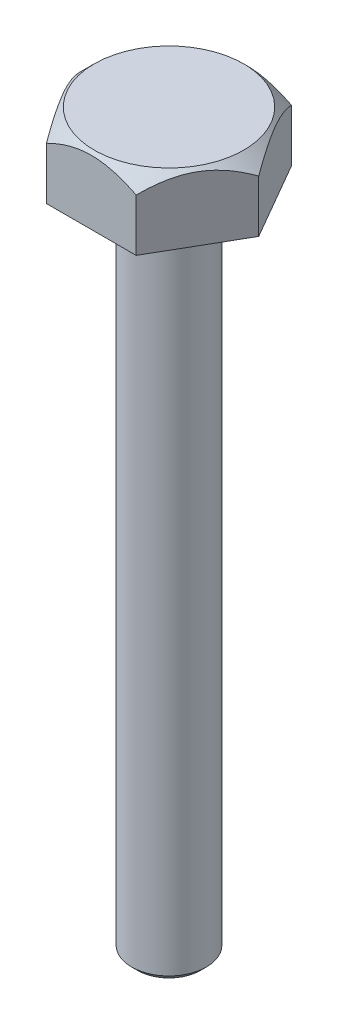
ISO-10303-21;
HEADER;
FILE_DESCRIPTION(('STEP AP214'),'2;1');
FILE_NAME('part.step','',(''),(''),'','','');
FILE_SCHEMA(('AUTOMOTIVE_DESIGN { 1 0 10303 214 1 1 1 1 }'));
ENDSEC;
DATA;
#1=APPLICATION_CONTEXT('core data for automotive mechanical design processes');
#2=APPLICATION_PROTOCOL_DEFINITION('international standard','automotive_design',2000,#1);
#3=PRODUCT_CONTEXT('',#1,'mechanical');
#4=PRODUCT('Part','Part','',(#3));
#5=PRODUCT_RELATED_PRODUCT_CATEGORY('part','',(#4));
#6=PRODUCT_DEFINITION_FORMATION('','',#4);
#7=PRODUCT_DEFINITION_CONTEXT('part definition',#1,'design');
#8=PRODUCT_DEFINITION('design','',#6,#7);
#9=PRODUCT_DEFINITION_SHAPE('','',#8);
#10=(LENGTH_UNIT() NAMED_UNIT(*) SI_UNIT(.MILLI.,.METRE.));
#11=(NAMED_UNIT(*) PLANE_ANGLE_UNIT() SI_UNIT($,.RADIAN.));
#12=(NAMED_UNIT(*) SI_UNIT($,.STERADIAN.) SOLID_ANGLE_UNIT());
#13=UNCERTAINTY_MEASURE_WITH_UNIT(LENGTH_MEASURE(1.E-05),#10,'distance_accuracy_value','');
#14=(GEOMETRIC_REPRESENTATION_CONTEXT(3) GLOBAL_UNCERTAINTY_ASSIGNED_CONTEXT((#13)) GLOBAL_UNIT_ASSIGNED_CONTEXT((#10,
#11,#12)) REPRESENTATION_CONTEXT('',''));
#15=CARTESIAN_POINT('',(0.,0.,0.));
#16=DIRECTION('',(0.,0.,1.));
#17=DIRECTION('',(1.,0.,0.));
#18=AXIS2_PLACEMENT_3D('',#15,#16,#17);
#19=CARTESIAN_POINT('',(30.0222139978612,-45.,51.9999999999998));
#20=DIRECTION('',(0.866025403784441,0.,0.499999999999995));
#21=DIRECTION('',(0.499999999999995,0.,-0.866025403784442));
#22=AXIS2_PLACEMENT_3D('',#19,#20,#21);
#23=PLANE('',#22);
#24=DIRECTION('',(0.,1.,0.));
#25=VECTOR('',#24,1.);
#26=CARTESIAN_POINT('',(60.0444279957212,-45.,0.));
#27=LINE('',#26,#25);
#28=CARTESIAN_POINT('',(60.0444279957212,-45.,0.));
#29=VERTEX_POINT('',#28);
#30=CARTESIAN_POINT('',(60.0444279957212,-10.0000000000014,0.));
#31=VERTEX_POINT('',#30);
#32=EDGE_CURVE('E126',#29,#31,#27,.T.);
#33=ORIENTED_EDGE('',*,*,#32,.T.);
#34=CARTESIAN_POINT('',(60.0445434657751,-10.0001154703869,-0.0002));
#35=CARTESIAN_POINT('',(59.7864654589408,-9.74204102394825,0.446804220153159));
#36=CARTESIAN_POINT('',(59.5273934547252,-9.4879536627119,0.895530094273221));
#37=CARTESIAN_POINT('',(59.007180391372,-8.98833098939079,1.79656555076206));
#38=CARTESIAN_POINT('',(58.7460392258412,-8.74279612061098,2.24887531740909));
#39=CARTESIAN_POINT('',(57.9591776962599,-8.01969424317608,3.61175946516538));
#40=CARTESIAN_POINT('',(57.4302681129248,-7.5558800497852,4.52785773611185));
#41=CARTESIAN_POINT('',(56.3606292168537,-6.66782291766471,6.38052664985892));
#42=CARTESIAN_POINT('',(55.8198495703374,-6.24382173529158,7.31718447332428));
#43=CARTESIAN_POINT('',(54.7294034599511,-5.44455349422062,9.20589253942921));
#44=CARTESIAN_POINT('',(54.1797383691726,-5.06927898510395,10.1579404038045));
#45=CARTESIAN_POINT('',(53.0804089118776,-4.37937556292623,12.0620348780967));
#46=CARTESIAN_POINT('',(52.5308802486714,-4.06388637101252,13.0138464429852));
#47=CARTESIAN_POINT('',(51.4240281951886,-3.49267453957314,14.9309704360794));
#48=CARTESIAN_POINT('',(50.8667044235457,-3.23695483511355,15.8962835248308));
#49=CARTESIAN_POINT('',(49.7467987752483,-2.79178958670772,17.8360170073652));
#50=CARTESIAN_POINT('',(49.1842323235144,-2.60218978873854,18.8104106844021));
#51=CARTESIAN_POINT('',(48.0543060242163,-2.2934501655637,20.7675004435948));
#52=CARTESIAN_POINT('',(47.4869469056895,-2.17429981294089,21.7501952630207));
#53=CARTESIAN_POINT('',(46.5113427741717,-2.03319122911529,23.4399911868836));
#54=CARTESIAN_POINT('',(46.1037295403586,-1.99322993327754,24.1459980176853));
#55=CARTESIAN_POINT('',(45.288020597666,-1.95167612563039,25.5588473506173));
#56=CARTESIAN_POINT('',(44.8799249140734,-1.95008168491468,26.2656898089493));
#57=CARTESIAN_POINT('',(44.0640057964976,-1.98529951069165,27.6789031754573));
#58=CARTESIAN_POINT('',(43.6561825137942,-2.02212562962843,28.3852738216091));
#59=CARTESIAN_POINT('',(42.8418298899032,-2.13363679445459,29.7957739414654));
#60=CARTESIAN_POINT('',(42.4353005710197,-2.20832248941607,30.4999033765379));
#61=CARTESIAN_POINT('',(41.623922764868,-2.39454189299686,31.9052509609266));
#62=CARTESIAN_POINT('',(41.2190765583396,-2.50611518507183,32.6064651598853));
#63=CARTESIAN_POINT('',(40.412216092256,-2.76451095087709,34.0039884817607));
#64=CARTESIAN_POINT('',(40.0102018479483,-2.9113336142421,34.7002975782681));
#65=CARTESIAN_POINT('',(39.2096518497491,-3.23827454574057,36.0868908491484));
#66=CARTESIAN_POINT('',(38.8111155333365,-3.41838732093504,36.7771759978363));
#67=CARTESIAN_POINT('',(38.017875656152,-3.80977115977922,38.1511077677096));
#68=CARTESIAN_POINT('',(37.6231724061646,-4.02104472782916,38.8347538506002));
#69=CARTESIAN_POINT('',(36.6070287630477,-4.60521339166235,40.594766268267));
#70=CARTESIAN_POINT('',(35.9887304273657,-5.00009639499698,41.6656903999035));
#71=CARTESIAN_POINT('',(34.7633032405128,-5.85344879079695,43.7881925485089));
#72=CARTESIAN_POINT('',(34.1561747269537,-6.31192010167665,44.8397699807171));
#73=CARTESIAN_POINT('',(32.9548834468553,-7.28227147123561,46.9204675125369));
#74=CARTESIAN_POINT('',(32.3606866497277,-7.79398356114847,47.9496465548567));
#75=CARTESIAN_POINT('',(31.4776043881334,-8.59647147709582,49.4791898992009));
#76=CARTESIAN_POINT('',(31.1846889985081,-8.86971037589588,49.9865342363506));
#77=CARTESIAN_POINT('',(30.6014667479989,-9.42700542859909,50.9967048063374));
#78=CARTESIAN_POINT('',(30.3111597002235,-9.71106079972311,51.4995313628796));
#79=CARTESIAN_POINT('',(30.0220985278074,-10.0001154703873,52.0001999999998));
#80=B_SPLINE_CURVE_WITH_KNOTS('',3,(#34,#35,#36,#37,#38,#39,#40,#41,#42,#43,#44,#45,#46,#47,#48,
#49,#50,#51,#52,#53,#54,#55,#56,#57,#58,#59,#60,#61,#62,#63,#64,#65,#66,#67,#68,#69,#70,#71,#72,
#73,#74,#75,#76,#77,#78,#79),.UNSPECIFIED.,.F.,.F.,(4,2,2,2,2,2,2,2,2,2,2,2,2,2,2,2,2,2,2,2,2,2,
4),(0.,1.73120255917824,3.46249471937635,6.92674897903945,10.410836798543,13.8943912642053,
17.3232079778031,20.7521930329857,24.1731240857036,27.5935438118118,30.0413233219973,
32.4889797690031,34.9375190179701,37.3861002466015,39.8373175810706,42.2885481029042,
44.7393745269946,47.1903980320212,51.0825946301753,54.974908678706,58.8552952790946,
60.7944610079078,62.7334866666266),.UNSPECIFIED.);
#81=CARTESIAN_POINT('',(30.0222139978612,-10.0000000000004,51.9999999999998));
#82=VERTEX_POINT('',#81);
#83=EDGE_CURVE('E60',#31,#82,#80,.T.);
#84=ORIENTED_EDGE('',*,*,#83,.T.);
#85=DIRECTION('',(0.,1.,0.));
#86=VECTOR('',#85,1.);
#87=CARTESIAN_POINT('',(30.0222139978612,-45.,51.9999999999998));
#88=LINE('',#87,#86);
#89=CARTESIAN_POINT('',(30.0222139978612,-45.,51.9999999999998));
#90=VERTEX_POINT('',#89);
#91=EDGE_CURVE('E64',#90,#82,#88,.T.);
#92=ORIENTED_EDGE('',*,*,#91,.F.);
#93=DIRECTION('',(0.499999999999995,0.,-0.866025403784442));
#94=VECTOR('',#93,1.);
#95=CARTESIAN_POINT('',(30.0222139978612,-45.,51.9999999999998));
#96=LINE('',#95,#94);
#97=EDGE_CURVE('E150',#90,#29,#96,.T.);
#98=ORIENTED_EDGE('',*,*,#97,.T.);
#99=EDGE_LOOP('',(#33,#84,#92,#98));
#100=FACE_BOUND('',#99,.T.);
#101=ADVANCED_FACE('F41',(#100),#23,.T.);
#102=CARTESIAN_POINT('',(-30.0222139978601,-45.,52.0000000000004));
#103=DIRECTION('',(0.,0.,1.));
#104=DIRECTION('',(1.,0.,0.));
#105=AXIS2_PLACEMENT_3D('',#102,#103,#104);
#106=PLANE('',#105);
#107=ORIENTED_EDGE('',*,*,#91,.T.);
#108=CARTESIAN_POINT('',(90.8938632440667,-54.6727834617611,51.9999999999992));
#109=CARTESIAN_POINT('',(89.5504864722996,-53.5067884121714,51.9999999999992));
#110=CARTESIAN_POINT('',(88.2039930705712,-52.3443708835845,51.9999999999992));
#111=CARTESIAN_POINT('',(85.5039309975092,-50.0277394466662,51.9999999999992));
#112=CARTESIAN_POINT('',(84.1503622105384,-48.8735256731456,51.9999999999992));
#113=CARTESIAN_POINT('',(81.4347136485867,-46.5738486041536,51.9999999999992));
#114=CARTESIAN_POINT('',(80.0726301741688,-45.4283896740304,51.9999999999993));
#115=CARTESIAN_POINT('',(77.3396021779961,-43.1480953330422,51.9999999999993));
#116=CARTESIAN_POINT('',(75.968657687125,-42.0132598851846,51.9999999999993));
#117=CARTESIAN_POINT('',(73.185415893131,-39.7300521772804,51.9999999999993));
#118=CARTESIAN_POINT('',(71.7728880995206,-38.5819606359992,51.9999999999994));
#119=CARTESIAN_POINT('',(68.9359443187834,-36.3005396584401,51.9999999999994));
#120=CARTESIAN_POINT('',(67.5115283063237,-35.1672102536324,51.9999999999994));
#121=CARTESIAN_POINT('',(64.6494837274142,-32.91804918836,51.9999999999994));
#122=CARTESIAN_POINT('',(63.2118584106515,-31.8022133978307,51.9999999999994));
#123=CARTESIAN_POINT('',(60.3210971698291,-29.5907906273971,51.9999999999995));
#124=CARTESIAN_POINT('',(58.8679612593283,-28.4952036297942,51.9999999999995));
#125=CARTESIAN_POINT('',(55.9419159848828,-26.3265853013323,51.9999999999995));
#126=CARTESIAN_POINT('',(54.4689828395049,-25.2535859926965,51.9999999999995));
#127=CARTESIAN_POINT('',(51.502512277947,-23.1363705697355,51.9999999999996));
#128=CARTESIAN_POINT('',(50.0089746315384,-22.0921547774204,51.9999999999996));
#129=CARTESIAN_POINT('',(46.996805849391,-20.0375584976056,51.9999999999996));
#130=CARTESIAN_POINT('',(45.4781541722698,-19.027207984574,51.9999999999996));
#131=CARTESIAN_POINT('',(43.1796128537923,-17.5435694706589,51.9999999999996));
#132=CARTESIAN_POINT('',(42.4099986030479,-17.054333890795,51.9999999999997));
#133=CARTESIAN_POINT('',(40.8634032398164,-16.0876603533286,51.9999999999997));
#134=CARTESIAN_POINT('',(40.0864222643945,-15.6102221768175,51.9999999999997));
#135=CARTESIAN_POINT('',(38.5304166005607,-14.6719589930306,51.9999999999997));
#136=CARTESIAN_POINT('',(37.7514508834595,-14.2110362854864,51.9999999999997));
#137=CARTESIAN_POINT('',(36.1852292133371,-13.3035272060015,51.9999999999997));
#138=CARTESIAN_POINT('',(35.397973481413,-12.8569404529963,51.9999999999997));
#139=CARTESIAN_POINT('',(33.814478702051,-11.9796354623624,51.9999999999997));
#140=CARTESIAN_POINT('',(33.018238142398,-11.5489199496323,51.9999999999998));
#141=CARTESIAN_POINT('',(31.4164102630234,-10.7052823627369,51.9999999999998));
#142=CARTESIAN_POINT('',(30.6108232701601,-10.2923596686977,51.9999999999998));
#143=CARTESIAN_POINT('',(28.9909279619983,-9.48691500383083,51.9999999999998));
#144=CARTESIAN_POINT('',(28.1766339356342,-9.09436440826349,51.9999999999998));
#145=CARTESIAN_POINT('',(26.5377992245099,-8.33132846994551,51.9999999999998));
#146=CARTESIAN_POINT('',(25.7132583192582,-7.96084360300037,51.9999999999998));
#147=CARTESIAN_POINT('',(23.2241791916238,-6.88642462741913,51.9999999999999));
#148=CARTESIAN_POINT('',(21.5433918050965,-6.21912680666249,51.9999999999999));
#149=CARTESIAN_POINT('',(18.9704946937658,-5.30192096749506,51.9999999999999));
#150=CARTESIAN_POINT('',(18.0941469020069,-5.00734056775779,51.9999999999999));
#151=CARTESIAN_POINT('',(16.3304304897878,-4.45311438614691,51.9999999999999));
#152=CARTESIAN_POINT('',(15.443062327066,-4.19346715856652,51.9999999999999));
#153=CARTESIAN_POINT('',(13.6580445184873,-3.71246570219744,52.));
#154=CARTESIAN_POINT('',(12.7603956314683,-3.49110866631926,52.));
#155=CARTESIAN_POINT('',(10.9558202502013,-3.08989470160482,52.));
#156=CARTESIAN_POINT('',(10.0488937167149,-2.91003794836363,52.));
#157=CARTESIAN_POINT('',(8.23297235277674,-2.59573942058979,52.));
#158=CARTESIAN_POINT('',(7.32402538061298,-2.46102242760543,52.));
#159=CARTESIAN_POINT('',(5.50044880642966,-2.23784575783965,52.));
#160=CARTESIAN_POINT('',(4.58581926214478,-2.14938561186587,52.));
#161=CARTESIAN_POINT('',(2.75323803859305,-2.02038759318325,52.0000000000001));
#162=CARTESIAN_POINT('',(1.83528661628648,-1.97984609003417,52.0000000000001));
#163=CARTESIAN_POINT('',(-0.0014803137554861,-1.94746418875032,52.0000000000001));
#164=CARTESIAN_POINT('',(-0.920295822166735,-1.95562382873903,52.0000000000001));
#165=CARTESIAN_POINT('',(-2.7575689607125,-2.0205320108917,52.0000000000001));
#166=CARTESIAN_POINT('',(-3.67602402316215,-2.07735284740119,52.0000000000001));
#167=CARTESIAN_POINT('',(-5.50872822957675,-2.23857876183826,52.0000000000001));
#168=CARTESIAN_POINT('',(-6.42297735802536,-2.34298401517021,52.0000000000002));
#169=CARTESIAN_POINT('',(-8.24519429376788,-2.59746666269973,52.0000000000002));
#170=CARTESIAN_POINT('',(-9.15316120156382,-2.74755046426637,52.0000000000002));
#171=CARTESIAN_POINT('',(-10.9608812749633,-3.0908077281104,52.0000000000002));
#172=CARTESIAN_POINT('',(-11.8606343617531,-3.28398160339682,52.0000000000002));
#173=CARTESIAN_POINT('',(-13.6568756349792,-3.71191051191629,52.0000000000002));
#174=CARTESIAN_POINT('',(-14.5532958301607,-3.94694970856731,52.0000000000002));
#175=CARTESIAN_POINT('',(-16.3355164562831,-4.45437230911218,52.0000000000003));
#176=CARTESIAN_POINT('',(-17.2213162468948,-4.7267579525208,52.0000000000003));
#177=CARTESIAN_POINT('',(-18.9816289041687,-5.3054704932223,52.0000000000003));
#178=CARTESIAN_POINT('',(-19.8561427926383,-5.6117942933954,52.0000000000003));
#179=CARTESIAN_POINT('',(-21.5937891086598,-6.25513051550924,52.0000000000003));
#180=CARTESIAN_POINT('',(-22.4569212527612,-6.59214370009087,52.0000000000003));
#181=CARTESIAN_POINT('',(-24.3605693993691,-7.37095216257304,52.0000000000003));
#182=CARTESIAN_POINT('',(-25.3983263981776,-7.81948637386516,52.0000000000004));
#183=CARTESIAN_POINT('',(-27.4576199763718,-8.75249539580748,52.0000000000004));
#184=CARTESIAN_POINT('',(-28.4791547131116,-9.2369742543672,52.0000000000004));
#185=CARTESIAN_POINT('',(-30.507208270308,-10.2375045095509,52.0000000000004));
#186=CARTESIAN_POINT('',(-31.5137196565872,-10.7535709322089,52.0000000000004));
#187=CARTESIAN_POINT('',(-33.512164725731,-11.8130484522965,52.0000000000004));
#188=CARTESIAN_POINT('',(-34.5040988715475,-12.3564586788914,52.0000000000005));
#189=CARTESIAN_POINT('',(-36.4764745459494,-13.4683136627819,52.0000000000005));
#190=CARTESIAN_POINT('',(-37.4568884841865,-14.0368072545755,52.0000000000005));
#191=CARTESIAN_POINT('',(-39.4052148777038,-15.1948027801057,52.0000000000005));
#192=CARTESIAN_POINT('',(-40.3731272437037,-15.7843048637619,52.0000000000005));
#193=CARTESIAN_POINT('',(-42.2972470872345,-16.9816124561098,52.0000000000005));
#194=CARTESIAN_POINT('',(-43.2534571155721,-17.5894138723483,52.0000000000005));
#195=CARTESIAN_POINT('',(-45.1553487881115,-18.8212428141494,52.0000000000006));
#196=CARTESIAN_POINT('',(-46.101030462716,-19.4452702928387,52.0000000000006));
#197=CARTESIAN_POINT('',(-47.9877868146267,-20.7110359246217,52.0000000000006));
#198=CARTESIAN_POINT('',(-48.928809917082,-21.3528508633096,52.0000000000006));
#199=CARTESIAN_POINT('',(-50.8019562536114,-22.6493259023017,52.0000000000006));
#200=CARTESIAN_POINT('',(-51.7340794840281,-23.3039860078841,52.0000000000006));
#201=CARTESIAN_POINT('',(-53.5902131492178,-24.6247468832788,52.0000000000006));
#202=CARTESIAN_POINT('',(-54.5142233823795,-25.2908479361941,52.0000000000007));
#203=CARTESIAN_POINT('',(-56.3548029151646,-26.6332593096256,52.0000000000007));
#204=CARTESIAN_POINT('',(-57.2713721397734,-27.3095697328688,52.0000000000007));
#205=CARTESIAN_POINT('',(-60.0087576325269,-29.3506026404731,52.0000000000007));
#206=CARTESIAN_POINT('',(-61.8194099905748,-30.728969932535,52.0000000000007));
#207=CARTESIAN_POINT('',(-65.4178182643262,-33.5151052064154,52.0000000000008));
#208=CARTESIAN_POINT('',(-67.2055746753492,-34.9228725504687,52.0000000000008));
#209=CARTESIAN_POINT('',(-69.9188996114158,-37.0895862575684,52.0000000000008));
#210=CARTESIAN_POINT('',(-70.851476317676,-37.8397798270726,52.0000000000008));
#211=CARTESIAN_POINT('',(-72.711694633653,-39.3462469302909,52.0000000000009));
#212=CARTESIAN_POINT('',(-73.6393362794022,-40.102520419512,52.0000000000009));
#213=CARTESIAN_POINT('',(-76.4158180634812,-42.3798907993665,52.0000000000009));
#214=CARTESIAN_POINT('',(-78.2578733410944,-43.9092640676019,52.0000000000009));
#215=CARTESIAN_POINT('',(-81.9063658376371,-46.9693729202027,52.0000000000009));
#216=CARTESIAN_POINT('',(-83.7129718426878,-48.4999075887176,52.000000000001));
#217=CARTESIAN_POINT('',(-86.4129861202291,-50.8068782513029,52.000000000001));
#218=CARTESIAN_POINT('',(-87.311245308278,-51.577646094416,52.000000000001));
#219=CARTESIAN_POINT('',(-89.1047542387976,-53.1226697377379,52.000000000001));
#220=CARTESIAN_POINT('',(-90.0000039909796,-53.8969255266724,52.000000000001));
#221=CARTESIAN_POINT('',(-90.8938632440656,-54.6727834617643,52.000000000001));
#222=B_SPLINE_CURVE_WITH_KNOTS('',3,(#108,#109,#110,#111,#112,#113,#114,#115,#116,#117,#118,
#119,#120,#121,#122,#123,#124,#125,#126,#127,#128,#129,#130,#131,#132,#133,#134,#135,#136,#137,
#138,#139,#140,#141,#142,#143,#144,#145,#146,#147,#148,#149,#150,#151,#152,#153,#154,#155,#156,
#157,#158,#159,#160,#161,#162,#163,#164,#165,#166,#167,#168,#169,#170,#171,#172,#173,#174,#175,
#176,#177,#178,#179,#180,#181,#182,#183,#184,#185,#186,#187,#188,#189,#190,#191,#192,#193,#194,
#195,#196,#197,#198,#199,#200,#201,#202,#203,#204,#205,#206,#207,#208,#209,#210,#211,#212,#213,
#214,#215,#216,#217,#218,#219,#220,#221),.UNSPECIFIED.,.F.,.F.,(4,2,2,2,2,2,2,2,2,2,2,2,2,2,2,2,
2,2,2,2,2,2,2,2,2,2,2,2,2,2,2,2,2,2,2,2,2,2,2,2,2,2,2,2,2,2,2,2,2,2,2,2,2,2,2,2,4),(0.,
5.33647077848684,10.6730290483922,16.0120942298001,21.3511408127576,26.8118373125386,
32.2725454516847,37.7319443460479,43.1913384683544,48.6580118451269,54.1247463544934,
59.5961981802856,62.3319697714796,65.0676905604675,67.782905772121,70.4980487506901,
73.2136557346523,75.9291680345071,78.6407553039375,81.3524010224423,86.7730328928577,
89.5460615467621,92.3189754037535,95.091685889621,97.8644081071028,100.619903535916,
103.375371014652,106.130629718665,108.885890579507,111.645251956449,114.404623504957,
117.164382291402,119.924167530673,122.703453114805,125.482905434359,128.262104315953,
131.041372280372,134.432187067909,137.823384293656,141.216207423338,144.60892256802,
148.008562644962,151.408226987078,154.807136596408,158.206036388159,161.623087877448,
165.04014077086,168.457278340452,171.874450316318,178.700836211937,185.527074178594,
189.117651431032,192.708202431391,199.890617453117,206.993846341314,210.544694111195,
214.095530411621),.UNSPECIFIED.);
#223=CARTESIAN_POINT('',(-30.0222139978601,-10.0000000000011,52.0000000000003));
#224=VERTEX_POINT('',#223);
#225=EDGE_CURVE('E114',#82,#224,#222,.T.);
#226=ORIENTED_EDGE('',*,*,#225,.T.);
#227=DIRECTION('',(0.,1.,0.));
#228=VECTOR('',#227,1.);
#229=CARTESIAN_POINT('',(-30.0222139978601,-45.,52.0000000000004));
#230=LINE('',#229,#228);
#231=CARTESIAN_POINT('',(-30.0222139978601,-45.,52.0000000000004));
#232=VERTEX_POINT('',#231);
#233=EDGE_CURVE('E115',#232,#224,#230,.T.);
#234=ORIENTED_EDGE('',*,*,#233,.F.);
#235=DIRECTION('',(1.,0.,0.));
#236=VECTOR('',#235,1.);
#237=CARTESIAN_POINT('',(-30.0222139978601,-45.,52.0000000000004));
#238=LINE('',#237,#236);
#239=EDGE_CURVE('E128',#232,#90,#238,.T.);
#240=ORIENTED_EDGE('',*,*,#239,.T.);
#241=EDGE_LOOP('',(#107,#226,#234,#240));
#242=FACE_BOUND('',#241,.T.);
#243=ADVANCED_FACE('F203',(#242),#106,.T.);
#244=CARTESIAN_POINT('',(-60.0444279957212,-45.,4.19287999697142E-13));
#245=DIRECTION('',(-0.866025403784435,0.,0.500000000000007));
#246=DIRECTION('',(0.500000000000007,0.,0.866025403784435));
#247=AXIS2_PLACEMENT_3D('',#244,#245,#246);
#248=PLANE('',#247);
#249=ORIENTED_EDGE('',*,*,#233,.T.);
#250=CARTESIAN_POINT('',(-30.0220985278063,-10.0001154703882,52.0002000000004));
#251=CARTESIAN_POINT('',(-30.2801765346406,-9.74204102394947,51.5531957798473));
#252=CARTESIAN_POINT('',(-30.5392485388562,-9.48795366271311,51.1044699057272));
#253=CARTESIAN_POINT('',(-31.0594616022094,-8.988330989392,50.2034344492384));
#254=CARTESIAN_POINT('',(-31.3206027677402,-8.74279612061217,49.7511246825913));
#255=CARTESIAN_POINT('',(-32.1074642973216,-8.01969424317726,48.388240534835));
#256=CARTESIAN_POINT('',(-32.6363738806567,-7.55588004978637,47.4721422638886));
#257=CARTESIAN_POINT('',(-33.7060127767278,-6.66782291766584,45.6194733501415));
#258=CARTESIAN_POINT('',(-34.2467924232441,-6.24382173529271,44.6828155266762));
#259=CARTESIAN_POINT('',(-35.3372385336304,-5.44455349422171,42.7941074605712));
#260=CARTESIAN_POINT('',(-35.8869036244089,-5.06927898510502,41.8420595961959));
#261=CARTESIAN_POINT('',(-36.986233081704,-4.37937556292727,39.9379651219038));
#262=CARTESIAN_POINT('',(-37.5357617449102,-4.06388637101355,38.9861535570153));
#263=CARTESIAN_POINT('',(-38.642613798393,-3.49267453957414,37.0690295639211));
#264=CARTESIAN_POINT('',(-39.199937570036,-3.23695483511453,36.1037164751697));
#265=CARTESIAN_POINT('',(-40.3198432183333,-2.79178958670868,34.1639829926353));
#266=CARTESIAN_POINT('',(-40.8824096700672,-2.60218978873949,33.1895893155984));
#267=CARTESIAN_POINT('',(-42.0123359693654,-2.29345016556464,31.2324995564057));
#268=CARTESIAN_POINT('',(-42.5796950878923,-2.17429981294183,30.2498047369798));
#269=CARTESIAN_POINT('',(-43.55529921941,-2.03319122911621,28.5600088131169));
#270=CARTESIAN_POINT('',(-43.9629124532231,-1.99322993327844,27.8540019823152));
#271=CARTESIAN_POINT('',(-44.7786213959157,-1.95167612563128,26.4411526493833));
#272=CARTESIAN_POINT('',(-45.1867170795084,-1.95008168491557,25.7343101910513));
#273=CARTESIAN_POINT('',(-46.0026361970842,-1.98529951069254,24.3210968245433));
#274=CARTESIAN_POINT('',(-46.4104594797875,-2.02212562962931,23.6147261783916));
#275=CARTESIAN_POINT('',(-47.2248121036785,-2.13363679445545,22.2042260585354));
#276=CARTESIAN_POINT('',(-47.631341422562,-2.20832248941693,21.5000966234629));
#277=CARTESIAN_POINT('',(-48.4427192287138,-2.3945418929977,20.0947490390742));
#278=CARTESIAN_POINT('',(-48.8475654352422,-2.50611518507267,19.3935348401155));
#279=CARTESIAN_POINT('',(-49.6544259013257,-2.76451095087792,17.9960115182402));
#280=CARTESIAN_POINT('',(-50.0564401456335,-2.91133361424291,17.2997024217328));
#281=CARTESIAN_POINT('',(-50.8569901438327,-3.23827454574136,15.9131091508526));
#282=CARTESIAN_POINT('',(-51.2555264602452,-3.41838732093582,15.2228240021647));
#283=CARTESIAN_POINT('',(-52.0487663374298,-3.80977115977999,13.8488922322914));
#284=CARTESIAN_POINT('',(-52.4434695874171,-4.02104472782991,13.1652461494008));
#285=CARTESIAN_POINT('',(-53.4596132305341,-4.60521339166312,11.405233731734));
#286=CARTESIAN_POINT('',(-54.0779115662162,-5.00009639499777,10.3343096000974));
#287=CARTESIAN_POINT('',(-55.3033387530692,-5.85344879079781,8.2118074514918));
#288=CARTESIAN_POINT('',(-55.9104672666284,-6.31192010167756,7.16023001928356));
#289=CARTESIAN_POINT('',(-57.1117585467269,-7.28227147123659,5.07953248746359));
#290=CARTESIAN_POINT('',(-57.7059553438545,-7.7939835611495,4.05035344514376));
#291=CARTESIAN_POINT('',(-58.5890376054489,-8.59647147709693,2.52081010079949));
#292=CARTESIAN_POINT('',(-58.8819529950742,-8.86971037589701,2.01346576364968));
#293=CARTESIAN_POINT('',(-59.4651752455835,-9.42700542860028,1.0032951936629));
#294=CARTESIAN_POINT('',(-59.7554822933589,-9.71106079972433,0.500468637120642));
#295=CARTESIAN_POINT('',(-60.0445434657751,-10.0001154703886,-0.000199999999581567));
#296=B_SPLINE_CURVE_WITH_KNOTS('',3,(#250,#251,#252,#253,#254,#255,#256,#257,#258,#259,#260,
#261,#262,#263,#264,#265,#266,#267,#268,#269,#270,#271,#272,#273,#274,#275,#276,#277,#278,#279,
#280,#281,#282,#283,#284,#285,#286,#287,#288,#289,#290,#291,#292,#293,#294,#295),.UNSPECIFIED.,
.F.,.F.,(4,2,2,2,2,2,2,2,2,2,2,2,2,2,2,2,2,2,2,2,2,2,4),(0.,1.73120255917825,3.46249471937637,
6.9267489790395,10.4108367985431,13.8943912642054,17.3232079778032,20.7521930329858,
24.1731240857038,27.5935438118119,30.0413233219975,32.4889797690032,34.9375190179701,
37.3861002466014,39.8373175810704,42.288548102904,44.7393745269944,47.1903980320209,
51.0825946301753,54.9749086787063,58.8552952790952,60.7944610079085,62.7334866666275),.UNSPECIFIED.);
#297=CARTESIAN_POINT('',(-60.044427995721,-10.0000000000014,0.));
#298=VERTEX_POINT('',#297);
#299=EDGE_CURVE('E98',#224,#298,#296,.T.);
#300=ORIENTED_EDGE('',*,*,#299,.T.);
#301=DIRECTION('',(0.,1.,0.));
#302=VECTOR('',#301,1.);
#303=CARTESIAN_POINT('',(-60.0444279957212,-45.,4.19287999697142E-13));
#304=LINE('',#303,#302);
#305=CARTESIAN_POINT('',(-60.0444279957212,-45.,4.19287999697142E-13));
#306=VERTEX_POINT('',#305);
#307=EDGE_CURVE('E109',#306,#298,#304,.T.);
#308=ORIENTED_EDGE('',*,*,#307,.F.);
#309=DIRECTION('',(0.500000000000007,0.,0.866025403784434));
#310=VECTOR('',#309,1.);
#311=CARTESIAN_POINT('',(-60.0444279957212,-45.,4.19287999697142E-13));
#312=LINE('',#311,#310);
#313=EDGE_CURVE('E138',#306,#232,#312,.T.);
#314=ORIENTED_EDGE('',*,*,#313,.T.);
#315=EDGE_LOOP('',(#249,#300,#308,#314));
#316=FACE_BOUND('',#315,.T.);
#317=ADVANCED_FACE('F107',(#316),#248,.T.);
#318=CARTESIAN_POINT('',(-30.0222139978609,-45.,-52.));
#319=DIRECTION('',(-0.866025403784442,0.,-0.499999999999995));
#320=DIRECTION('',(-0.499999999999995,0.,0.866025403784442));
#321=AXIS2_PLACEMENT_3D('',#318,#319,#320);
#322=PLANE('',#321);
#323=ORIENTED_EDGE('',*,*,#307,.T.);
#324=CARTESIAN_POINT('',(-60.0445434657751,-10.0001154703886,0.000200000000419288));
#325=CARTESIAN_POINT('',(-59.7864654589408,-9.74204102394989,-0.446804220152739));
#326=CARTESIAN_POINT('',(-59.5273934547252,-9.48795366271352,-0.895530094272799));
#327=CARTESIAN_POINT('',(-59.007180391372,-8.98833098939239,-1.79656555076164));
#328=CARTESIAN_POINT('',(-58.7460392258412,-8.74279612061256,-2.24887531740867));
#329=CARTESIAN_POINT('',(-57.9591776962599,-8.01969424317761,-3.61175946516495));
#330=CARTESIAN_POINT('',(-57.4302681129248,-7.55588004978671,-4.52785773611142));
#331=CARTESIAN_POINT('',(-56.3606292168536,-6.66782291766615,-6.3805266498585));
#332=CARTESIAN_POINT('',(-55.8198495703374,-6.243821735293,-7.31718447332387));
#333=CARTESIAN_POINT('',(-54.7294034599511,-5.44455349422198,-9.2058925394288));
#334=CARTESIAN_POINT('',(-54.1797383691726,-5.06927898510527,-10.1579404038041));
#335=CARTESIAN_POINT('',(-53.0804089118775,-4.37937556292748,-12.0620348780963));
#336=CARTESIAN_POINT('',(-52.5308802486714,-4.06388637101375,-13.0138464429848));
#337=CARTESIAN_POINT('',(-51.4240281951885,-3.4926745395743,-14.930970436079));
#338=CARTESIAN_POINT('',(-50.8667044235456,-3.23695483511468,-15.8962835248305));
#339=CARTESIAN_POINT('',(-49.7467987752483,-2.7917895867088,-17.8360170073648));
#340=CARTESIAN_POINT('',(-49.1842323235144,-2.6021897887396,-18.8104106844017));
#341=CARTESIAN_POINT('',(-48.0543060242162,-2.29345016556472,-20.7675004435944));
#342=CARTESIAN_POINT('',(-47.4869469056894,-2.17429981294189,-21.7501952630204));
#343=CARTESIAN_POINT('',(-46.5113427741717,-2.03319122911625,-23.4399911868833));
#344=CARTESIAN_POINT('',(-46.1037295403586,-1.99322993327847,-24.145998017685));
#345=CARTESIAN_POINT('',(-45.288020597666,-1.95167612563128,-25.5588473506169));
#346=CARTESIAN_POINT('',(-44.8799249140734,-1.95008168491557,-26.2656898089489));
#347=CARTESIAN_POINT('',(-44.0640057964976,-1.98529951069251,-27.6789031754569));
#348=CARTESIAN_POINT('',(-43.6561825137942,-2.02212562962928,-28.3852738216086));
#349=CARTESIAN_POINT('',(-42.8418298899032,-2.1336367944554,-29.7957739414649));
#350=CARTESIAN_POINT('',(-42.4353005710198,-2.20832248941687,-30.4999033765374));
#351=CARTESIAN_POINT('',(-41.623922764868,-2.39454189299762,-31.9052509609261));
#352=CARTESIAN_POINT('',(-41.2190765583396,-2.50611518507258,-32.6064651598847));
#353=CARTESIAN_POINT('',(-40.4122160922561,-2.76451095087781,-34.0039884817601));
#354=CARTESIAN_POINT('',(-40.0102018479484,-2.91133361424279,-34.7002975782676));
#355=CARTESIAN_POINT('',(-39.2096518497492,-3.23827454574122,-36.0868908491477));
#356=CARTESIAN_POINT('',(-38.8111155333366,-3.41838732093567,-36.7771759978357));
#357=CARTESIAN_POINT('',(-38.0178756561521,-3.80977115977982,-38.1511077677089));
#358=CARTESIAN_POINT('',(-37.6231724061648,-4.02104472782973,-38.8347538505996));
#359=CARTESIAN_POINT('',(-36.6070287630478,-4.60521339166291,-40.5947662682664));
#360=CARTESIAN_POINT('',(-35.9887304273657,-5.00009639499755,-41.6656903999029));
#361=CARTESIAN_POINT('',(-34.7633032405127,-5.85344879079756,-43.7881925485086));
#362=CARTESIAN_POINT('',(-34.1561747269536,-6.31192010167728,-44.8397699807168));
#363=CARTESIAN_POINT('',(-32.9548834468552,-7.28227147123628,-46.9204675125368));
#364=CARTESIAN_POINT('',(-32.3606866497275,-7.79398356114917,-47.9496465548566));
#365=CARTESIAN_POINT('',(-31.4776043881331,-8.59647147709657,-49.4791898992009));
#366=CARTESIAN_POINT('',(-31.1846889985078,-8.86971037589664,-49.9865342363507));
#367=CARTESIAN_POINT('',(-30.6014667479985,-9.42700542859989,-50.9967048063375));
#368=CARTESIAN_POINT('',(-30.3111597002232,-9.71106079972394,-51.4995313628798));
#369=CARTESIAN_POINT('',(-30.022098527807,-10.0001154703882,-52.0002));
#370=B_SPLINE_CURVE_WITH_KNOTS('',3,(#324,#325,#326,#327,#328,#329,#330,#331,#332,#333,#334,
#335,#336,#337,#338,#339,#340,#341,#342,#343,#344,#345,#346,#347,#348,#349,#350,#351,#352,#353,
#354,#355,#356,#357,#358,#359,#360,#361,#362,#363,#364,#365,#366,#367,#368,#369),.UNSPECIFIED.,
.F.,.F.,(4,2,2,2,2,2,2,2,2,2,2,2,2,2,2,2,2,2,2,2,2,2,4),(0.,1.73120255917825,3.46249471937639,
6.92674897903953,10.4108367985431,13.8943912642055,17.3232079778033,20.7521930329859,
24.1731240857039,27.5935438118121,30.0413233219976,32.4889797690033,34.9375190179703,
37.3861002466016,39.8373175810706,42.2885481029042,44.7393745269945,47.190398032021,
51.0825946301754,54.9749086787064,58.8552952790953,60.7944610079086,62.7334866666275),.UNSPECIFIED.);
#371=CARTESIAN_POINT('',(-30.0222139978606,-10.0000000000011,-51.9999999999999));
#372=VERTEX_POINT('',#371);
#373=EDGE_CURVE('E94',#298,#372,#370,.T.);
#374=ORIENTED_EDGE('',*,*,#373,.T.);
#375=DIRECTION('',(0.,1.,0.));
#376=VECTOR('',#375,1.);
#377=CARTESIAN_POINT('',(-30.0222139978609,-45.,-52.));
#378=LINE('',#377,#376);
#379=CARTESIAN_POINT('',(-30.0222139978609,-45.,-52.));
#380=VERTEX_POINT('',#379);
#381=EDGE_CURVE('E119',#380,#372,#378,.T.);
#382=ORIENTED_EDGE('',*,*,#381,.F.);
#383=DIRECTION('',(-0.499999999999995,0.,0.866025403784442));
#384=VECTOR('',#383,1.);
#385=CARTESIAN_POINT('',(-30.0222139978609,-45.,-52.));
#386=LINE('',#385,#384);
#387=EDGE_CURVE('E118',#380,#306,#386,.T.);
#388=ORIENTED_EDGE('',*,*,#387,.T.);
#389=EDGE_LOOP('',(#323,#374,#382,#388));
#390=FACE_BOUND('',#389,.T.);
#391=ADVANCED_FACE('F117',(#390),#322,.T.);
#392=CARTESIAN_POINT('',(30.0222139978605,-45.,-52.0000000000002));
#393=DIRECTION('',(0.,0.,-1.));
#394=DIRECTION('',(-1.,0.,0.));
#395=AXIS2_PLACEMENT_3D('',#392,#393,#394);
#396=PLANE('',#395);
#397=ORIENTED_EDGE('',*,*,#381,.T.);
#398=CARTESIAN_POINT('',(-90.8938632440663,-54.6727834617644,-51.9999999999998));
#399=CARTESIAN_POINT('',(-89.5504864722992,-53.5067884121747,-51.9999999999998));
#400=CARTESIAN_POINT('',(-88.2039930705709,-52.3443708835877,-51.9999999999998));
#401=CARTESIAN_POINT('',(-85.5039309975089,-50.0277394466693,-51.9999999999998));
#402=CARTESIAN_POINT('',(-84.1503622105381,-48.8735256731487,-51.9999999999998));
#403=CARTESIAN_POINT('',(-81.4347136485864,-46.5738486041565,-51.9999999999998));
#404=CARTESIAN_POINT('',(-80.0726301741685,-45.4283896740333,-51.9999999999998));
#405=CARTESIAN_POINT('',(-77.3396021779958,-43.148095333045,-51.9999999999998));
#406=CARTESIAN_POINT('',(-75.9686576871248,-42.0132598851873,-51.9999999999998));
#407=CARTESIAN_POINT('',(-73.1854158931308,-39.730052177283,-51.9999999999999));
#408=CARTESIAN_POINT('',(-71.7728880995204,-38.5819606360018,-51.9999999999999));
#409=CARTESIAN_POINT('',(-68.9359443187833,-36.3005396584426,-51.9999999999999));
#410=CARTESIAN_POINT('',(-67.5115283063236,-35.1672102536349,-51.9999999999999));
#411=CARTESIAN_POINT('',(-64.649483727414,-32.9180491883624,-51.9999999999999));
#412=CARTESIAN_POINT('',(-63.2118584106513,-31.802213397833,-51.9999999999999));
#413=CARTESIAN_POINT('',(-60.321097169829,-29.5907906273993,-51.9999999999999));
#414=CARTESIAN_POINT('',(-58.8679612593282,-28.4952036297964,-51.9999999999999));
#415=CARTESIAN_POINT('',(-55.9419159848828,-26.3265853013343,-51.9999999999999));
#416=CARTESIAN_POINT('',(-54.4689828395048,-25.2535859926985,-51.9999999999999));
#417=CARTESIAN_POINT('',(-51.502512277947,-23.1363705697373,-51.9999999999999));
#418=CARTESIAN_POINT('',(-50.0089746315384,-22.0921547774222,-51.9999999999999));
#419=CARTESIAN_POINT('',(-46.996805849391,-20.0375584976073,-52.));
#420=CARTESIAN_POINT('',(-45.4781541722698,-19.0272079845756,-52.));
#421=CARTESIAN_POINT('',(-43.1796128537924,-17.5435694706605,-52.));
#422=CARTESIAN_POINT('',(-42.409998603048,-17.0543338907965,-52.));
#423=CARTESIAN_POINT('',(-40.8634032398165,-16.08766035333,-52.));
#424=CARTESIAN_POINT('',(-40.0864222643946,-15.6102221768189,-52.));
#425=CARTESIAN_POINT('',(-38.5304166005607,-14.671958993032,-52.));
#426=CARTESIAN_POINT('',(-37.7514508834596,-14.2110362854878,-52.));
#427=CARTESIAN_POINT('',(-36.1852292133372,-13.3035272060028,-52.));
#428=CARTESIAN_POINT('',(-35.3979734814131,-12.8569404529976,-52.));
#429=CARTESIAN_POINT('',(-33.8144787020511,-11.9796354623636,-52.));
#430=CARTESIAN_POINT('',(-33.0182381423981,-11.5489199496335,-52.));
#431=CARTESIAN_POINT('',(-31.4164102630235,-10.705282362738,-52.));
#432=CARTESIAN_POINT('',(-30.6108232701602,-10.2923596686988,-52.));
#433=CARTESIAN_POINT('',(-28.9909279619984,-9.48691500383188,-52.));
#434=CARTESIAN_POINT('',(-28.1766339356343,-9.09436440826451,-52.));
#435=CARTESIAN_POINT('',(-26.53779922451,-8.33132846994646,-52.));
#436=CARTESIAN_POINT('',(-25.7132583192583,-7.9608436030013,-52.));
#437=CARTESIAN_POINT('',(-23.2241791916239,-6.88642462741997,-52.));
#438=CARTESIAN_POINT('',(-21.5433918050966,-6.21912680666326,-52.));
#439=CARTESIAN_POINT('',(-18.9704946937659,-5.30192096749574,-52.));
#440=CARTESIAN_POINT('',(-18.094146902007,-5.00734056775843,-52.));
#441=CARTESIAN_POINT('',(-16.3304304897879,-4.45311438614749,-52.));
#442=CARTESIAN_POINT('',(-15.4430623270662,-4.19346715856707,-52.));
#443=CARTESIAN_POINT('',(-13.6580445184874,-3.71246570219792,-52.0000000000001));
#444=CARTESIAN_POINT('',(-12.7603956314684,-3.4911086663197,-52.0000000000001));
#445=CARTESIAN_POINT('',(-10.9558202502014,-3.0898947016052,-52.0000000000001));
#446=CARTESIAN_POINT('',(-10.048893716715,-2.91003794836398,-52.0000000000001));
#447=CARTESIAN_POINT('',(-8.23297235277682,-2.59573942059007,-52.0000000000001));
#448=CARTESIAN_POINT('',(-7.32402538061305,-2.46102242760568,-52.0000000000001));
#449=CARTESIAN_POINT('',(-5.50044880642973,-2.23784575783984,-52.0000000000001));
#450=CARTESIAN_POINT('',(-4.58581926214485,-2.14938561186603,-52.0000000000001));
#451=CARTESIAN_POINT('',(-2.7532380385931,-2.02038759318335,-52.0000000000001));
#452=CARTESIAN_POINT('',(-1.83528661628653,-1.97984609003425,-52.0000000000001));
#453=CARTESIAN_POINT('',(0.00148031375546713,-1.94746418875034,-52.0000000000001));
#454=CARTESIAN_POINT('',(0.920295822166727,-1.955623828739,-52.0000000000001));
#455=CARTESIAN_POINT('',(2.75756896071251,-2.02053201089161,-52.0000000000001));
#456=CARTESIAN_POINT('',(3.67602402316218,-2.07735284740108,-52.0000000000001));
#457=CARTESIAN_POINT('',(5.50872822957681,-2.23857876183809,-52.0000000000001));
#458=CARTESIAN_POINT('',(6.42297735802543,-2.34298401517002,-52.0000000000001));
#459=CARTESIAN_POINT('',(8.24519429376798,-2.5974666626995,-52.0000000000001));
#460=CARTESIAN_POINT('',(9.15316120156394,-2.74755046426612,-52.0000000000001));
#461=CARTESIAN_POINT('',(10.9608812749634,-3.0908077281101,-52.0000000000001));
#462=CARTESIAN_POINT('',(11.8606343617532,-3.28398160339648,-52.0000000000001));
#463=CARTESIAN_POINT('',(13.6568756349794,-3.7119105119159,-52.0000000000002));
#464=CARTESIAN_POINT('',(14.5532958301609,-3.94694970856691,-52.0000000000002));
#465=CARTESIAN_POINT('',(16.3355164562833,-4.45437230911175,-52.0000000000002));
#466=CARTESIAN_POINT('',(17.2213162468951,-4.72675795252034,-52.0000000000002));
#467=CARTESIAN_POINT('',(18.981628904169,-5.30547049322179,-52.0000000000002));
#468=CARTESIAN_POINT('',(19.8561427926386,-5.61179429339488,-52.0000000000002));
#469=CARTESIAN_POINT('',(21.5937891086601,-6.25513051550869,-52.0000000000002));
#470=CARTESIAN_POINT('',(22.4569212527616,-6.59214370009029,-52.0000000000002));
#471=CARTESIAN_POINT('',(24.3605693993695,-7.37095216257242,-52.0000000000002));
#472=CARTESIAN_POINT('',(25.398326398178,-7.8194863738645,-52.0000000000002));
#473=CARTESIAN_POINT('',(27.4576199763722,-8.75249539580676,-52.0000000000002));
#474=CARTESIAN_POINT('',(28.4791547131121,-9.23697425436647,-52.0000000000002));
#475=CARTESIAN_POINT('',(30.5072082703084,-10.2375045095501,-52.0000000000002));
#476=CARTESIAN_POINT('',(31.5137196565876,-10.7535709322081,-52.0000000000002));
#477=CARTESIAN_POINT('',(33.5121647257314,-11.8130484522956,-52.0000000000002));
#478=CARTESIAN_POINT('',(34.5040988715479,-12.3564586788905,-52.0000000000002));
#479=CARTESIAN_POINT('',(36.4764745459499,-13.468313662781,-52.0000000000002));
#480=CARTESIAN_POINT('',(37.456888484187,-14.0368072545745,-52.0000000000002));
#481=CARTESIAN_POINT('',(39.4052148777043,-15.1948027801046,-52.0000000000002));
#482=CARTESIAN_POINT('',(40.3731272437042,-15.7843048637608,-52.0000000000002));
#483=CARTESIAN_POINT('',(42.297247087235,-16.9816124561086,-52.0000000000002));
#484=CARTESIAN_POINT('',(43.2534571155726,-17.5894138723471,-52.0000000000003));
#485=CARTESIAN_POINT('',(45.155348788112,-18.8212428141482,-52.0000000000003));
#486=CARTESIAN_POINT('',(46.1010304627165,-19.4452702928374,-52.0000000000003));
#487=CARTESIAN_POINT('',(47.9877868146272,-20.7110359246203,-52.0000000000003));
#488=CARTESIAN_POINT('',(48.9288099170826,-21.3528508633082,-52.0000000000003));
#489=CARTESIAN_POINT('',(50.8019562536119,-22.6493259023003,-52.0000000000003));
#490=CARTESIAN_POINT('',(51.7340794840287,-23.3039860078827,-52.0000000000003));
#491=CARTESIAN_POINT('',(53.5902131492184,-24.6247468832773,-52.0000000000003));
#492=CARTESIAN_POINT('',(54.5142233823801,-25.2908479361925,-52.0000000000003));
#493=CARTESIAN_POINT('',(56.3548029151652,-26.633259309624,-52.0000000000003));
#494=CARTESIAN_POINT('',(57.2713721397741,-27.3095697328672,-52.0000000000003));
#495=CARTESIAN_POINT('',(60.0087576325276,-29.3506026404714,-52.0000000000003));
#496=CARTESIAN_POINT('',(61.8194099905755,-30.7289699325332,-52.0000000000003));
#497=CARTESIAN_POINT('',(65.4178182643269,-33.5151052064135,-52.0000000000003));
#498=CARTESIAN_POINT('',(67.2055746753499,-34.9228725504668,-52.0000000000003));
#499=CARTESIAN_POINT('',(69.9188996114165,-37.0895862575663,-52.0000000000003));
#500=CARTESIAN_POINT('',(70.8514763176767,-37.8397798270705,-52.0000000000003));
#501=CARTESIAN_POINT('',(72.7116946336537,-39.3462469302887,-52.0000000000003));
#502=CARTESIAN_POINT('',(73.6393362794029,-40.1025204195097,-52.0000000000003));
#503=CARTESIAN_POINT('',(76.4158180634818,-42.3798907993641,-52.0000000000004));
#504=CARTESIAN_POINT('',(78.257873341095,-43.9092640675993,-52.0000000000004));
#505=CARTESIAN_POINT('',(81.9063658376376,-46.9693729202,-52.0000000000004));
#506=CARTESIAN_POINT('',(83.7129718426883,-48.4999075887147,-52.0000000000004));
#507=CARTESIAN_POINT('',(86.4129861202296,-50.8068782512999,-52.0000000000004));
#508=CARTESIAN_POINT('',(87.3112453082784,-51.5776460944129,-52.0000000000004));
#509=CARTESIAN_POINT('',(89.104754238798,-53.1226697377348,-52.0000000000004));
#510=CARTESIAN_POINT('',(90.00000399098,-53.8969255266692,-52.0000000000004));
#511=CARTESIAN_POINT('',(90.893863244066,-54.672783461761,-52.0000000000004));
#512=B_SPLINE_CURVE_WITH_KNOTS('',3,(#398,#399,#400,#401,#402,#403,#404,#405,#406,#407,#408,
#409,#410,#411,#412,#413,#414,#415,#416,#417,#418,#419,#420,#421,#422,#423,#424,#425,#426,#427,
#428,#429,#430,#431,#432,#433,#434,#435,#436,#437,#438,#439,#440,#441,#442,#443,#444,#445,#446,
#447,#448,#449,#450,#451,#452,#453,#454,#455,#456,#457,#458,#459,#460,#461,#462,#463,#464,#465,
#466,#467,#468,#469,#470,#471,#472,#473,#474,#475,#476,#477,#478,#479,#480,#481,#482,#483,#484,
#485,#486,#487,#488,#489,#490,#491,#492,#493,#494,#495,#496,#497,#498,#499,#500,#501,#502,#503,
#504,#505,#506,#507,#508,#509,#510,#511),.UNSPECIFIED.,.F.,.F.,(4,2,2,2,2,2,2,2,2,2,2,2,2,2,2,2,
2,2,2,2,2,2,2,2,2,2,2,2,2,2,2,2,2,2,2,2,2,2,2,2,2,2,2,2,2,2,2,2,2,2,2,2,2,2,2,2,4),(0.,
5.33647077848691,10.6730290483923,16.0120942298003,21.3511408127579,26.8118373125389,
32.2725454516851,37.7319443460483,43.1913384683549,48.6580118451275,54.124746354494,
59.5961981802864,62.3319697714803,65.0676905604682,67.7829057721218,70.498048750691,
73.2136557346531,75.929168034508,78.6407553039384,81.3524010224433,86.7730328928588,
89.5460615467632,92.3189754037546,95.0916858896221,97.864408107104,100.619903535918,
103.375371014653,106.130629718666,108.885890579508,111.645251956451,114.404623504958,
117.164382291403,119.924167530674,122.703453114807,125.48290543436,128.262104315954,
131.041372280374,134.43218706791,137.823384293658,141.21620742334,144.608922568022,
148.008562644963,151.408226987079,154.80713659641,158.206036388161,161.62308787745,
165.040140770862,168.457278340453,171.874450316319,178.700836211938,185.527074178595,
189.117651431033,192.708202431392,199.890617453118,206.993846341314,210.544694111195,
214.095530411621),.UNSPECIFIED.);
#513=CARTESIAN_POINT('',(30.0222139978606,-10.0000000000004,-52.0000000000001));
#514=VERTEX_POINT('',#513);
#515=EDGE_CURVE('E101',#372,#514,#512,.T.);
#516=ORIENTED_EDGE('',*,*,#515,.T.);
#517=DIRECTION('',(0.,1.,0.));
#518=VECTOR('',#517,1.);
#519=CARTESIAN_POINT('',(30.0222139978605,-45.,-52.0000000000002));
#520=LINE('',#519,#518);
#521=CARTESIAN_POINT('',(30.0222139978605,-45.,-52.0000000000002));
#522=VERTEX_POINT('',#521);
#523=EDGE_CURVE('E125',#522,#514,#520,.T.);
#524=ORIENTED_EDGE('',*,*,#523,.F.);
#525=DIRECTION('',(-1.,0.,0.));
#526=VECTOR('',#525,1.);
#527=CARTESIAN_POINT('',(30.0222139978605,-45.,-52.0000000000002));
#528=LINE('',#527,#526);
#529=EDGE_CURVE('E143',#522,#380,#528,.T.);
#530=ORIENTED_EDGE('',*,*,#529,.T.);
#531=EDGE_LOOP('',(#397,#516,#524,#530));
#532=FACE_BOUND('',#531,.T.);
#533=ADVANCED_FACE('F202',(#532),#396,.T.);
#534=CARTESIAN_POINT('',(60.0444279957212,-45.,0.));
#535=DIRECTION('',(0.866025403784438,0.,-0.500000000000001));
#536=DIRECTION('',(-0.500000000000001,0.,-0.866025403784438));
#537=AXIS2_PLACEMENT_3D('',#534,#535,#536);
#538=PLANE('',#537);
#539=ORIENTED_EDGE('',*,*,#523,.T.);
#540=CARTESIAN_POINT('',(30.0220985278067,-10.0001154703873,-52.0002000000002));
#541=CARTESIAN_POINT('',(30.280176534641,-9.74204102394864,-51.553195779847));
#542=CARTESIAN_POINT('',(30.5392485388566,-9.48795366271228,-51.104469905727));
#543=CARTESIAN_POINT('',(31.0594616022098,-8.98833098939115,-50.2034344492381));
#544=CARTESIAN_POINT('',(31.3206027677405,-8.74279612061133,-49.7511246825911));
#545=CARTESIAN_POINT('',(32.1074642973219,-8.01969424317639,-48.3882405348348));
#546=CARTESIAN_POINT('',(32.636373880657,-7.55588004978549,-47.4721422638883));
#547=CARTESIAN_POINT('',(33.7060127767282,-6.66782291766494,-45.6194733501413));
#548=CARTESIAN_POINT('',(34.2467924232445,-6.24382173529179,-44.6828155266759));
#549=CARTESIAN_POINT('',(35.3372385336308,-5.44455349422078,-42.794107460571));
#550=CARTESIAN_POINT('',(35.8869036244093,-5.06927898510407,-41.8420595961956));
#551=CARTESIAN_POINT('',(36.9862330817043,-4.3793755629263,-39.9379651219035));
#552=CARTESIAN_POINT('',(37.5357617449105,-4.06388637101259,-38.986153557015));
#553=CARTESIAN_POINT('',(38.6426137983934,-3.49267453957315,-37.0690295639207));
#554=CARTESIAN_POINT('',(39.1999375700363,-3.23695483511352,-36.1037164751693));
#555=CARTESIAN_POINT('',(40.3198432183336,-2.79178958670765,-34.1639829926349));
#556=CARTESIAN_POINT('',(40.8824096700676,-2.60218978873846,-33.189589315598));
#557=CARTESIAN_POINT('',(42.0123359693657,-2.29345016556359,-31.2324995564053));
#558=CARTESIAN_POINT('',(42.5796950878926,-2.17429981294075,-30.2498047369793));
#559=CARTESIAN_POINT('',(43.5552992194103,-2.03319122911512,-28.5600088131164));
#560=CARTESIAN_POINT('',(43.9629124532234,-1.99322993327736,-27.8540019823147));
#561=CARTESIAN_POINT('',(44.7786213959161,-1.95167612563019,-26.4411526493828));
#562=CARTESIAN_POINT('',(45.1867170795087,-1.95008168491447,-25.7343101910508));
#563=CARTESIAN_POINT('',(46.0026361970845,-1.98529951069142,-24.3210968245427));
#564=CARTESIAN_POINT('',(46.4104594797878,-2.02212562962819,-23.614726178391));
#565=CARTESIAN_POINT('',(47.2248121036789,-2.13363679445432,-22.2042260585347));
#566=CARTESIAN_POINT('',(47.6313414225623,-2.20832248941579,-21.5000966234622));
#567=CARTESIAN_POINT('',(48.4427192287141,-2.39454189299656,-20.0947490390735));
#568=CARTESIAN_POINT('',(48.8475654352425,-2.50611518507152,-19.3935348401148));
#569=CARTESIAN_POINT('',(49.6544259013261,-2.76451095087676,-17.9960115182394));
#570=CARTESIAN_POINT('',(50.0564401456338,-2.91133361424175,-17.299702421732));
#571=CARTESIAN_POINT('',(50.8569901438331,-3.2382745457402,-15.9131091508518));
#572=CARTESIAN_POINT('',(51.2555264602456,-3.41838732093466,-15.2228240021638));
#573=CARTESIAN_POINT('',(52.0487663374302,-3.80977115977882,-13.8488922322905));
#574=CARTESIAN_POINT('',(52.4434695874175,-4.02104472782874,-13.1652461493999));
#575=CARTESIAN_POINT('',(53.4596132305345,-4.60521339166192,-11.4052337317331));
#576=CARTESIAN_POINT('',(54.0779115662165,-5.00009639499655,-10.3343096000966));
#577=CARTESIAN_POINT('',(55.3033387530695,-5.85344879079651,-8.21180745149108));
#578=CARTESIAN_POINT('',(55.9104672666286,-6.31192010167621,-7.16023001928287));
#579=CARTESIAN_POINT('',(57.111758546727,-7.28227147123517,-5.07953248746299));
#580=CARTESIAN_POINT('',(57.7059553438547,-7.79398356114805,-4.0503534451432));
#581=CARTESIAN_POINT('',(58.589037605449,-8.5964714770954,-2.52081010079898));
#582=CARTESIAN_POINT('',(58.8819529950743,-8.86971037589545,-2.01346576364919));
#583=CARTESIAN_POINT('',(59.4651752455836,-9.42700542859866,-1.00329519366244));
#584=CARTESIAN_POINT('',(59.7554822933589,-9.7110607997227,-0.500468637120201));
#585=CARTESIAN_POINT('',(60.0445434657751,-10.0001154703869,0.000200000000000302));
#586=B_SPLINE_CURVE_WITH_KNOTS('',3,(#540,#541,#542,#543,#544,#545,#546,#547,#548,#549,#550,
#551,#552,#553,#554,#555,#556,#557,#558,#559,#560,#561,#562,#563,#564,#565,#566,#567,#568,#569,
#570,#571,#572,#573,#574,#575,#576,#577,#578,#579,#580,#581,#582,#583,#584,#585),.UNSPECIFIED.,
.F.,.F.,(4,2,2,2,2,2,2,2,2,2,2,2,2,2,2,2,2,2,2,2,2,2,4),(0.,1.73120255917826,3.4624947193764,
6.92674897903956,10.4108367985432,13.8943912642055,17.3232079778034,20.752193032986,
24.173124085704,27.5935438118122,30.0413233219978,32.4889797690035,34.9375190179706,
37.3861002466019,39.837317581071,42.2885481029046,44.739374526995,47.1903980320216,
51.0825946301758,54.9749086787067,58.8552952790954,60.7944610079086,62.7334866666274),.UNSPECIFIED.);
#587=EDGE_CURVE('E174',#514,#31,#586,.T.);
#588=ORIENTED_EDGE('',*,*,#587,.T.);
#589=ORIENTED_EDGE('',*,*,#32,.F.);
#590=DIRECTION('',(-0.500000000000001,0.,-0.866025403784438));
#591=VECTOR('',#590,1.);
#592=CARTESIAN_POINT('',(60.0444279957212,-45.,0.));
#593=LINE('',#592,#591);
#594=EDGE_CURVE('E145',#29,#522,#593,.T.);
#595=ORIENTED_EDGE('',*,*,#594,.T.);
#596=EDGE_LOOP('',(#539,#588,#589,#595));
#597=FACE_BOUND('',#596,.T.);
#598=ADVANCED_FACE('F208',(#597),#538,.T.);
#599=CARTESIAN_POINT('',(0.,-45.,0.));
#600=DIRECTION('',(0.,1.,0.));
#601=DIRECTION('',(0.,0.,1.));
#602=AXIS2_PLACEMENT_3D('',#599,#600,#601);
#603=PLANE('',#602);
#604=CARTESIAN_POINT('',(0.,-45.,0.));
#605=DIRECTION('',(0.,1.,0.));
#606=DIRECTION('',(0.,0.,1.));
#607=AXIS2_PLACEMENT_3D('',#604,#605,#606);
#608=CIRCLE('',#607,25.);
#609=CARTESIAN_POINT('',(0.,-45.,25.));
#610=VERTEX_POINT('',#609);
#611=EDGE_CURVE('E230',#610,#610,#608,.T.);
#612=ORIENTED_EDGE('',*,*,#611,.T.);
#613=EDGE_LOOP('',(#612));
#614=FACE_BOUND('',#613,.T.);
#615=ORIENTED_EDGE('',*,*,#97,.F.);
#616=ORIENTED_EDGE('',*,*,#239,.F.);
#617=ORIENTED_EDGE('',*,*,#313,.F.);
#618=ORIENTED_EDGE('',*,*,#387,.F.);
#619=ORIENTED_EDGE('',*,*,#529,.F.);
#620=ORIENTED_EDGE('',*,*,#594,.F.);
#621=EDGE_LOOP('',(#615,#616,#617,#618,#619,#620));
#622=FACE_BOUND('',#621,.T.);
#623=ADVANCED_FACE('F170',(#614,#622),#603,.F.);
#624=CARTESIAN_POINT('',(0.,-5.94188426188681E-13,0.));
#625=DIRECTION('',(0.,-1.,0.));
#626=DIRECTION('',(1.,0.,0.));
#627=AXIS2_PLACEMENT_3D('',#624,#625,#626);
#628=CONICAL_SURFACE('',#627,50.0444279957212,0.785398163397437);
#629=ORIENTED_EDGE('',*,*,#587,.F.);
#630=ORIENTED_EDGE('',*,*,#515,.F.);
#631=ORIENTED_EDGE('',*,*,#373,.F.);
#632=ORIENTED_EDGE('',*,*,#299,.F.);
#633=ORIENTED_EDGE('',*,*,#225,.F.);
#634=ORIENTED_EDGE('',*,*,#83,.F.);
#635=EDGE_LOOP('',(#629,#630,#631,#632,#633,#634));
#636=FACE_BOUND('',#635,.T.);
#637=CARTESIAN_POINT('',(0.,-5.94188426188681E-13,0.));
#638=DIRECTION('',(0.,1.,0.));
#639=DIRECTION('',(-1.,0.,0.));
#640=AXIS2_PLACEMENT_3D('',#637,#638,#639);
#641=CIRCLE('',#640,50.0444279957212);
#642=CARTESIAN_POINT('',(-50.0444279957212,-1.18837685237736E-12,0.));
#643=VERTEX_POINT('',#642);
#644=EDGE_CURVE('E223',#643,#643,#641,.T.);
#645=ORIENTED_EDGE('',*,*,#644,.F.);
#646=EDGE_LOOP('',(#645));
#647=FACE_BOUND('',#646,.T.);
#648=ADVANCED_FACE('F96',(#636,#647),#628,.T.);
#649=CARTESIAN_POINT('',(0.,0.,0.));
#650=DIRECTION('',(0.,1.,0.));
#651=DIRECTION('',(0.,0.,1.));
#652=AXIS2_PLACEMENT_3D('',#649,#650,#651);
#653=PLANE('',#652);
#654=ORIENTED_EDGE('',*,*,#644,.T.);
#655=EDGE_LOOP('',(#654));
#656=FACE_BOUND('',#655,.T.);
#657=ADVANCED_FACE('F167',(#656),#653,.T.);
#658=CARTESIAN_POINT('',(0.,-490.,0.));
#659=DIRECTION('',(0.,1.,0.));
#660=DIRECTION('',(0.,0.,1.));
#661=AXIS2_PLACEMENT_3D('',#658,#659,#660);
#662=CYLINDRICAL_SURFACE('',#661,25.);
#663=CARTESIAN_POINT('',(0.,-486.,0.));
#664=DIRECTION('',(0.,1.,0.));
#665=DIRECTION('',(0.,0.,1.));
#666=AXIS2_PLACEMENT_3D('',#663,#664,#665);
#667=CIRCLE('',#666,25.);
#668=CARTESIAN_POINT('',(0.,-486.,25.));
#669=VERTEX_POINT('',#668);
#670=EDGE_CURVE('E49',#669,#669,#667,.T.);
#671=ORIENTED_EDGE('',*,*,#670,.T.);
#672=EDGE_LOOP('',(#671));
#673=FACE_BOUND('',#672,.T.);
#674=ORIENTED_EDGE('',*,*,#611,.F.);
#675=EDGE_LOOP('',(#674));
#676=FACE_BOUND('',#675,.T.);
#677=ADVANCED_FACE('F169',(#673,#676),#662,.T.);
#678=CARTESIAN_POINT('',(0.,-490.,0.));
#679=DIRECTION('',(0.,1.,0.));
#680=DIRECTION('',(0.,0.,1.));
#681=AXIS2_PLACEMENT_3D('',#678,#679,#680);
#682=PLANE('',#681);
#683=CARTESIAN_POINT('',(0.,-490.,0.));
#684=DIRECTION('',(0.,1.,0.));
#685=DIRECTION('',(0.,0.,1.));
#686=AXIS2_PLACEMENT_3D('',#683,#684,#685);
#687=CIRCLE('',#686,21.0000000000001);
#688=CARTESIAN_POINT('',(0.,-490.,21.0000000000001));
#689=VERTEX_POINT('',#688);
#690=EDGE_CURVE('E11',#689,#689,#687,.F.);
#691=ORIENTED_EDGE('',*,*,#690,.T.);
#692=EDGE_LOOP('',(#691));
#693=FACE_BOUND('',#692,.T.);
#694=ADVANCED_FACE('F234',(#693),#682,.F.);
#695=CARTESIAN_POINT('',(0.,-486.,0.));
#696=DIRECTION('',(0.,1.,0.));
#697=DIRECTION('',(0.,0.,1.));
#698=AXIS2_PLACEMENT_3D('',#695,#696,#697);
#699=CONICAL_SURFACE('',#698,25.,0.785398163397453);
#700=ORIENTED_EDGE('',*,*,#690,.F.);
#701=EDGE_LOOP('',(#700));
#702=FACE_BOUND('',#701,.T.);
#703=ORIENTED_EDGE('',*,*,#670,.F.);
#704=EDGE_LOOP('',(#703));
#705=FACE_BOUND('',#704,.T.);
#706=ADVANCED_FACE('F42',(#702,#705),#699,.T.);
#707=CLOSED_SHELL('',(#101,#243,#317,#391,#533,#598,#623,#648,#657,#677,#694,#706));
#708=MANIFOLD_SOLID_BREP('B2',#707);
#709=ADVANCED_BREP_SHAPE_REPRESENTATION('',(#18,#708),#14);
#710=SHAPE_DEFINITION_REPRESENTATION(#9,#709);
ENDSEC;
END-ISO-10303-21;
